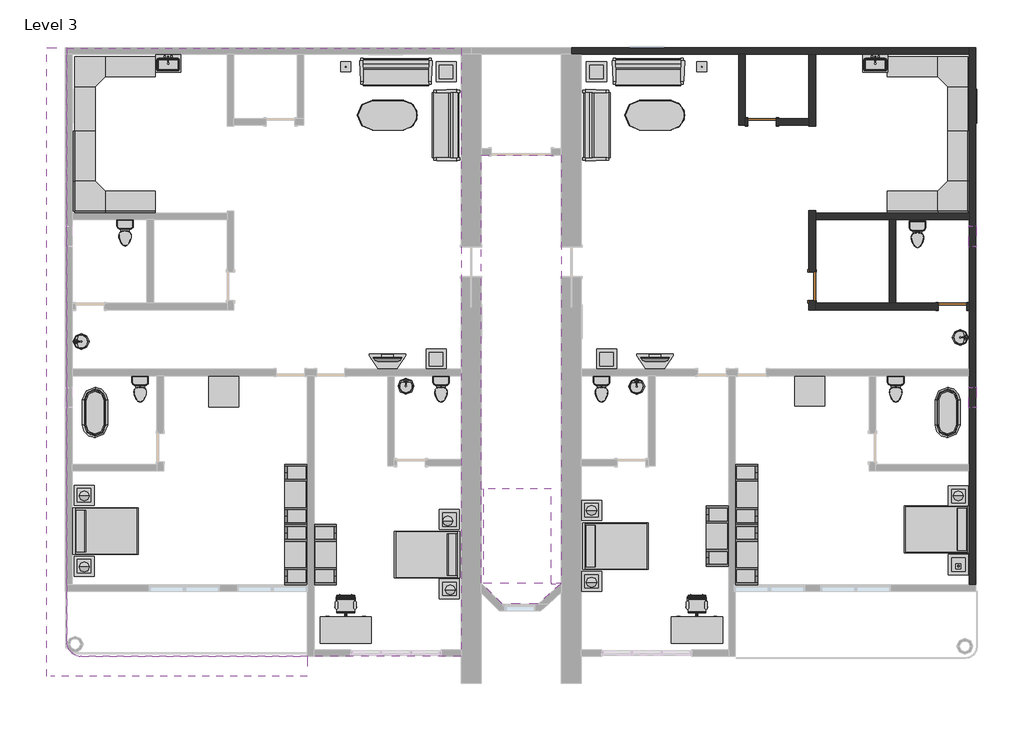
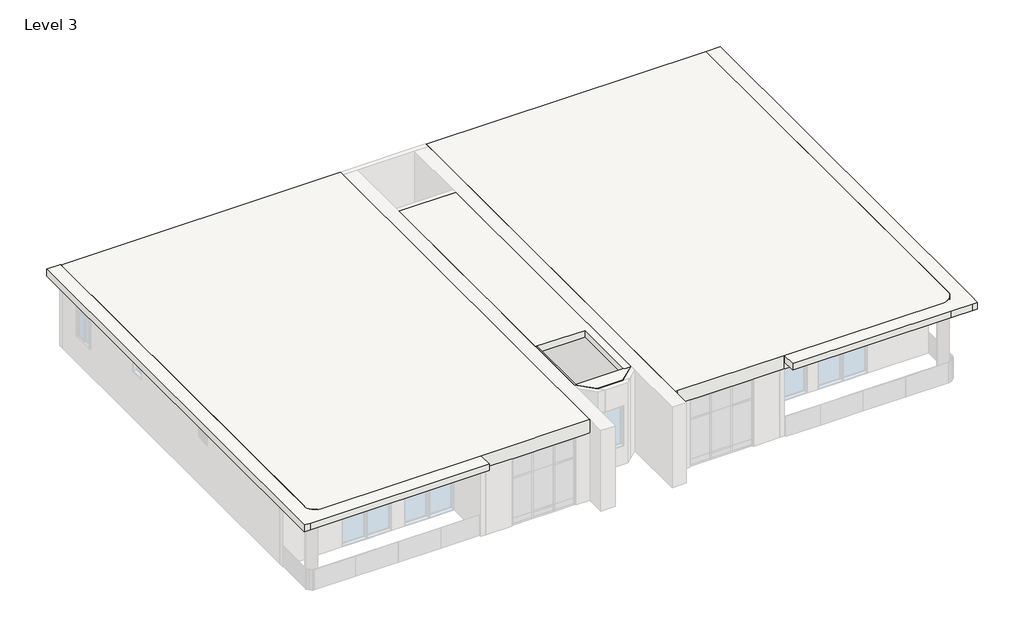
# One storey, part 3 of 3: 42 furniture elements, 14 flow terminals, 10 light fixtures, 9 walls, 4 slabs, 3 doors, 3 windows.
"""IFC4 building model written with IfcOpenShell, lengths in millimetres."""

from ifc_helpers import new_model, si_unit, point, frame, frame_2d, origin, place, context, project, spatial, polyline, circle_curve, trimmed, segment, composite_curve, outline, extrude, faceted_brep, transform, mapped, element, save
from components import door_2703ae13, door_10fd3a06, flow_terminal_38af2918, flow_terminal_d49f872f, toilet_domestic_3d_toilet_domestic_3d_f7549cf7, toilet_domestic_3d_toilet_domestic_3d_183bbd19, flow_terminal_b374fae2, furniture_07436f11, furniture_096e7f55, chair_task_arms_chair_task_arms_fa5a08ef, furniture_072f6425, furniture_cf0b6580, furniture_aff9b2fb, furniture_56245f3a, tv_stand_tv_stand_6ce107e5, furniture_b5c51a22, furniture_2c34a4f9, furniture_4d44e21c, furniture_45e3acac, light_fixture_100w_120v_8564026f, table_lamp_hemispheric_60w_120v_02721d88, window_0038ecf3, window_54100e87

model = new_model("IFC4")

# Units and contexts
model_context = context("Model", 3, world=origin())
ifc_project = project(units=[si_unit("LENGTHUNIT", "METRE", prefix="MILLI")], contexts=[model_context])

# Site, building, storey
site = spatial("IfcSite", under=ifc_project)
building = spatial("IfcBuilding", under=site)
storey = spatial("IfcBuildingStorey", under=building, Name="Level 3", Elevation=7315.2)

# Doors
placement = place(None, origin())
door_shape = door_2703ae13(model_context)
element("IfcDoor", 1, ObjectType="Door-Single-Panel.0001 : 34\" x 80\"", at=placement, inside=storey, context=model_context, shape_type="MappedRepresentation", body=[
    mapped(door_shape, transform((2528.3512296, 9464.0758558, 7315.2), x_axis=(-1.0, 0.0, 0.0), y_axis=(0.0, -1.0, 0.0), z_axis=(0.0, 0.0, 1.0))),
])
door_2_shape = door_10fd3a06(model_context)
element("IfcDoor", 2, ObjectType="Door-Single-Panel.0001 : 34\" x 80\"", at=placement, inside=storey, context=model_context, shape_type="MappedRepresentation", body=[
    mapped(door_2_shape, transform((8319.5512296, 3850.6758558, 7315.2), x_axis=(1.0, 0.0, 0.0), y_axis=(0.0, 1.0, 0.0), z_axis=(0.0, 0.0, 1.0))),
])
element("IfcDoor", 3, ObjectType="Door-Single-Panel.0001 : 34\" x 80\"", at=placement, inside=storey, context=model_context, shape_type="MappedRepresentation", body=[
    mapped(door_2_shape, transform((4052.3512296, 4460.2758558, 7315.2), x_axis=(0.0, -1.0, 0.0), y_axis=(1.0, 0.0, 0.0), z_axis=(0.0, 0.0, 1.0))),
])

# Flow terminals
flow_terminal_shape = flow_terminal_38af2918(model_context)
element("IfcFlowTerminal", 4, ObjectType="Sink Kitchen-Single : 30\" x 21\"", at=placement, inside=storey, context=model_context, shape_type="MappedRepresentation", body=[
    mapped(flow_terminal_shape, transform((-15534.038011, 11239.7304546, 7315.2), x_axis=(1.0, 0.0, 0.0), y_axis=(0.0, 1.0, 0.0), z_axis=(0.0, 0.0, 1.0))),
])
element("IfcFlowTerminal", 5, ObjectType="Sink Kitchen-Single : 30\" x 21\"", at=placement, inside=storey, context=model_context, shape_type="MappedRepresentation", body=[
    mapped(flow_terminal_shape, transform((5954.361989, 11239.7304546, 7315.2), x_axis=(1.0, 0.0, 0.0), y_axis=(0.0, 1.0, 0.0), z_axis=(0.0, 0.0, 1.0))),
])
flow_terminal_2_shape = flow_terminal_d49f872f(model_context)
element("IfcFlowTerminal", 6, ObjectType="Sink Vanity-Round : 19\" x 19\"", at=placement, inside=storey, context=model_context, shape_type="MappedRepresentation", body=[
    mapped(flow_terminal_2_shape, transform((-18078.2570794, 2687.2241152, 7315.2), x_axis=(0.0, 1.0, 0.0), y_axis=(-1.0, 0.0, 0.0), z_axis=(0.0, 0.0, 1.0))),
])
element("IfcFlowTerminal", 7, ObjectType="Sink Vanity-Round : 19\" x 19\"", at=placement, inside=storey, context=model_context, shape_type="MappedRepresentation", body=[
    mapped(flow_terminal_2_shape, transform((8468.5749463, 3007.5275963, 7315.2), x_axis=(0.0, -1.0, 0.0), y_axis=(1.0, 0.0, 0.0), z_axis=(0.0, 0.0, 1.0))),
])
element("IfcFlowTerminal", 8, ObjectType="Sink Vanity-Round : 19\" x 19\"", at=placement, inside=storey, context=model_context, shape_type="MappedRepresentation", body=[
    mapped(flow_terminal_2_shape, transform((-8388.700511, 1341.8921141, 7315.2), x_axis=(1.0, 0.0, 0.0), y_axis=(0.0, 1.0, 0.0), z_axis=(0.0, 0.0, 1.0))),
])
element("IfcFlowTerminal", 9, ObjectType="Sink Vanity-Round : 19\" x 19\"", at=placement, inside=storey, context=model_context, shape_type="MappedRepresentation", body=[
    mapped(flow_terminal_2_shape, transform((-1378.300511, 1331.0855344, 7315.2), x_axis=(1.0, 0.0, 0.0), y_axis=(0.0, 1.0, 0.0), z_axis=(0.0, 0.0, 1.0))),
])
toilet_domestic_3d_toilet_domestic_3d_shape = toilet_domestic_3d_toilet_domestic_3d_f7549cf7(model_context)
toilet_domestic_3d_toilet_domestic_3d_2_shape = toilet_domestic_3d_toilet_domestic_3d_183bbd19(model_context)
element("IfcFlowTerminal", 10, ObjectType="Toilet-Domestic-3D : Toilet-Domestic-3D", at=placement, inside=storey, context=model_context, shape_type="MappedRepresentation", body=[
    mapped(toilet_domestic_3d_toilet_domestic_3d_shape, transform((6592.3512296, 1247.7798284, 7315.2), x_axis=(1.0, 0.0, 0.0), y_axis=(0.0, 1.0, 0.0), z_axis=(0.0, 0.0, 1.0))),
    mapped(toilet_domestic_3d_toilet_domestic_3d_2_shape, transform((6592.3512296, 1247.7798284, 7315.2), x_axis=(1.0, 0.0, 0.0), y_axis=(0.0, 1.0, 0.0), z_axis=(0.0, 0.0, 1.0))),
])
element("IfcFlowTerminal", 11, ObjectType="Toilet-Domestic-3D : Toilet-Domestic-3D", at=placement, inside=storey, context=model_context, shape_type="MappedRepresentation", body=[
    mapped(toilet_domestic_3d_toilet_domestic_3d_shape, transform((-2348.4487704, 1247.7798284, 7315.2), x_axis=(1.0, 0.0, 0.0), y_axis=(0.0, 1.0, 0.0), z_axis=(0.0, 0.0, 1.0))),
    mapped(toilet_domestic_3d_toilet_domestic_3d_2_shape, transform((-2348.4487704, 1247.7798284, 7315.2), x_axis=(1.0, 0.0, 0.0), y_axis=(0.0, 1.0, 0.0), z_axis=(0.0, 0.0, 1.0))),
])
element("IfcFlowTerminal", 12, ObjectType="Toilet-Domestic-3D : Toilet-Domestic-3D", at=placement, inside=storey, context=model_context, shape_type="MappedRepresentation", body=[
    mapped(toilet_domestic_3d_toilet_domestic_3d_shape, transform((-16369.2487704, 1247.7798284, 7315.2), x_axis=(1.0, 0.0, 0.0), y_axis=(0.0, 1.0, 0.0), z_axis=(0.0, 0.0, 1.0))),
    mapped(toilet_domestic_3d_toilet_domestic_3d_2_shape, transform((-16369.2487704, 1247.7798284, 7315.2), x_axis=(1.0, 0.0, 0.0), y_axis=(0.0, 1.0, 0.0), z_axis=(0.0, 0.0, 1.0))),
])
element("IfcFlowTerminal", 13, ObjectType="Toilet-Domestic-3D : Toilet-Domestic-3D", at=placement, inside=storey, context=model_context, shape_type="MappedRepresentation", body=[
    mapped(toilet_domestic_3d_toilet_domestic_3d_shape, transform((-16826.4487704, 5997.5798284, 7315.2), x_axis=(1.0, 0.0, 0.0), y_axis=(0.0, 1.0, 0.0), z_axis=(0.0, 0.0, 1.0))),
    mapped(toilet_domestic_3d_toilet_domestic_3d_2_shape, transform((-16826.4487704, 5997.5798284, 7315.2), x_axis=(1.0, 0.0, 0.0), y_axis=(0.0, 1.0, 0.0), z_axis=(0.0, 0.0, 1.0))),
])
element("IfcFlowTerminal", 14, ObjectType="Toilet-Domestic-3D : Toilet-Domestic-3D", at=placement, inside=storey, context=model_context, shape_type="MappedRepresentation", body=[
    mapped(toilet_domestic_3d_toilet_domestic_3d_shape, transform((7252.7512296, 5946.7798284, 7315.2), x_axis=(1.0, 0.0, 0.0), y_axis=(0.0, 1.0, 0.0), z_axis=(0.0, 0.0, 1.0))),
    mapped(toilet_domestic_3d_toilet_domestic_3d_2_shape, transform((7252.7512296, 5946.7798284, 7315.2), x_axis=(1.0, 0.0, 0.0), y_axis=(0.0, 1.0, 0.0), z_axis=(0.0, 0.0, 1.0))),
])
element("IfcFlowTerminal", 15, ObjectType="Toilet-Domestic-3D : Toilet-Domestic-3D", at=placement, inside=storey, context=model_context, shape_type="MappedRepresentation", body=[
    mapped(toilet_domestic_3d_toilet_domestic_3d_shape, transform((-7225.2487704, 1247.7798284, 7315.2), x_axis=(1.0, 0.0, 0.0), y_axis=(0.0, 1.0, 0.0), z_axis=(0.0, 0.0, 1.0))),
    mapped(toilet_domestic_3d_toilet_domestic_3d_2_shape, transform((-7225.2487704, 1247.7798284, 7315.2), x_axis=(1.0, 0.0, 0.0), y_axis=(0.0, 1.0, 0.0), z_axis=(0.0, 0.0, 1.0))),
])
flow_terminal_3_shape = flow_terminal_b374fae2(model_context)
element("IfcFlowTerminal", 16, ObjectType="Tub-Free Standing-3D : 30\" x 60\"", at=placement, inside=storey, context=model_context, shape_type="MappedRepresentation", body=[
    mapped(flow_terminal_3_shape, transform((-17740.8487704, 624.8758558, 7315.2), x_axis=(1.0, 0.0, 0.0), y_axis=(0.0, 1.0, 0.0), z_axis=(0.0, 0.0, 1.0))),
])
element("IfcFlowTerminal", 17, ObjectType="Tub-Free Standing-3D : 30\" x 60\"", at=placement, inside=storey, context=model_context, shape_type="MappedRepresentation", body=[
    mapped(flow_terminal_3_shape, transform((8167.1512296, 624.8758558, 7315.2), x_axis=(1.0, 0.0, 0.0), y_axis=(0.0, 1.0, 0.0), z_axis=(0.0, 0.0, 1.0))),
])

# Furniture
furniture_shape = furniture_07436f11(model_context)
element("IfcFurniture", 18, ObjectType="96\" x 96\"", at=placement, inside=storey, context=model_context, shape_type="MappedRepresentation", body=[
    mapped(furniture_shape, transform((-18269.5170182, 11991.0988634, 7315.2), x_axis=(1.0, 0.0, 0.0), y_axis=(0.0, 1.0, 0.0), z_axis=(0.0, 0.0, 1.0))),
])
element("IfcFurniture", 19, ObjectType="96\" x 96\"", at=placement, inside=storey, context=model_context, shape_type="MappedRepresentation", body=[
    mapped(furniture_shape, transform((9322.5742372, 11364.3441035, 7315.2), x_axis=(0.0, -1.0, 0.0), y_axis=(1.0, 0.0, 0.0), z_axis=(0.0, 0.0, 1.0))),
])
furniture_2_shape = furniture_096e7f55(model_context)
element("IfcFurniture", 20, ObjectType="Bed-Shaker : Double 56\" x 78\"", at=placement, inside=storey, context=model_context, shape_type="MappedRepresentation", body=[
    mapped(furniture_2_shape, transform((-18401.2487704, -2962.8741442, 7315.2), x_axis=(0.0, 1.0, 0.0), y_axis=(-1.0, 0.0, 0.0), z_axis=(0.0, 0.0, 1.0))),
])
element("IfcFurniture", 21, ObjectType="Bed-Shaker : Double 56\" x 78\"", at=placement, inside=storey, context=model_context, shape_type="MappedRepresentation", body=[
    mapped(furniture_2_shape, transform((-6666.4487704, -3712.1741442, 7315.2), x_axis=(0.0, -1.0, 0.0), y_axis=(1.0, 0.0, 0.0), z_axis=(0.0, 0.0, 1.0))),
])
element("IfcFurniture", 22, ObjectType="Bed-Shaker : Double 56\" x 78\"", at=placement, inside=storey, context=model_context, shape_type="MappedRepresentation", body=[
    mapped(furniture_2_shape, transform((-2907.2487704, -3420.0741442, 7315.2), x_axis=(0.0, 1.0, 0.0), y_axis=(-1.0, 0.0, 0.0), z_axis=(0.0, 0.0, 1.0))),
])
element("IfcFurniture", 23, ObjectType="Bed-Shaker : Double 56\" x 78\"", at=placement, inside=storey, context=model_context, shape_type="MappedRepresentation", body=[
    mapped(furniture_2_shape, transform((8827.5512296, -2950.1741442, 7315.2), x_axis=(0.0, -1.0, 0.0), y_axis=(1.0, 0.0, 0.0), z_axis=(0.0, 0.0, 1.0))),
])
chair_task_arms_chair_task_arms_shape = chair_task_arms_chair_task_arms_fa5a08ef(model_context)
element("IfcFurniture", 24, ObjectType="Chair-Task Arms : Chair-Task Arms", at=placement, inside=storey, context=model_context, shape_type="MappedRepresentation", body=[
    mapped(chair_task_arms_chair_task_arms_shape, transform((688.1420493, -5184.3566833, 7315.2), x_axis=(-1.0, 0.0, 0.0), y_axis=(0.0, -1.0, 0.0), z_axis=(0.0, 0.0, 1.0))),
])
element("IfcFurniture", 25, ObjectType="Chair-Task Arms : Chair-Task Arms", at=placement, inside=storey, context=model_context, shape_type="MappedRepresentation", body=[
    mapped(chair_task_arms_chair_task_arms_shape, transform((-9979.8579507, -5184.3566833, 7315.2), x_axis=(-1.0, 0.0, 0.0), y_axis=(0.0, -1.0, 0.0), z_axis=(0.0, 0.0, 1.0))),
])
furniture_3_shape = furniture_072f6425(model_context)
element("IfcFurniture", 26, ObjectType="Desk : 60\" x 30\"", at=placement, inside=storey, context=model_context, shape_type="MappedRepresentation", body=[
    mapped(furniture_3_shape, transform((-10882.8487704, -6371.702585, 7315.2), x_axis=(1.0, 0.0, 0.0), y_axis=(0.0, 1.0, 0.0), z_axis=(0.0, 0.0, 1.0))),
])
element("IfcFurniture", 27, ObjectType="Desk : 60\" x 30\"", at=placement, inside=storey, context=model_context, shape_type="MappedRepresentation", body=[
    mapped(furniture_3_shape, transform((-214.8487704, -6371.702585, 7315.2), x_axis=(1.0, 0.0, 0.0), y_axis=(0.0, 1.0, 0.0), z_axis=(0.0, 0.0, 1.0))),
])
furniture_4_shape = furniture_cf0b6580(model_context)
element("IfcFurniture", 28, ObjectType="Entertainment Center : 72\" x 72\" x 24\"", at=placement, inside=storey, context=model_context, shape_type="MappedRepresentation", body=[
    mapped(furniture_4_shape, transform((1613.9512296, -3134.3241442, 7315.2), x_axis=(0.0, -1.0, 0.0), y_axis=(1.0, 0.0, 0.0), z_axis=(0.0, 0.0, 1.0))),
])
element("IfcFurniture", 29, ObjectType="Entertainment Center : 72\" x 72\" x 24\"", at=placement, inside=storey, context=model_context, shape_type="MappedRepresentation", body=[
    mapped(furniture_4_shape, transform((1613.9512296, -3693.1241442, 7315.2), x_axis=(0.0, 1.0, 0.0), y_axis=(-1.0, 0.0, 0.0), z_axis=(0.0, 0.0, 1.0))),
])
element("IfcFurniture", 30, ObjectType="Entertainment Center : 72\" x 72\" x 24\"", at=placement, inside=storey, context=model_context, shape_type="MappedRepresentation", body=[
    mapped(furniture_4_shape, transform((1613.9512296, -1864.3241442, 7315.2), x_axis=(0.0, 1.0, 0.0), y_axis=(-1.0, 0.0, 0.0), z_axis=(0.0, 0.0, 1.0))),
])
element("IfcFurniture", 31, ObjectType="Entertainment Center : 72\" x 72\" x 24\"", at=placement, inside=storey, context=model_context, shape_type="MappedRepresentation", body=[
    mapped(furniture_4_shape, transform((-11187.6487704, -3693.1241442, 7315.2), x_axis=(0.0, -1.0, 0.0), y_axis=(1.0, 0.0, 0.0), z_axis=(0.0, 0.0, 1.0))),
])
element("IfcFurniture", 32, ObjectType="Entertainment Center : 72\" x 72\" x 24\"", at=placement, inside=storey, context=model_context, shape_type="MappedRepresentation", body=[
    mapped(furniture_4_shape, transform((-11187.6487704, -1864.3241442, 7315.2), x_axis=(0.0, -1.0, 0.0), y_axis=(1.0, 0.0, 0.0), z_axis=(0.0, 0.0, 1.0))),
])
element("IfcFurniture", 33, ObjectType="Entertainment Center : 72\" x 72\" x 24\"", at=placement, inside=storey, context=model_context, shape_type="MappedRepresentation", body=[
    mapped(furniture_4_shape, transform((-11187.6487704, -3693.1241442, 7315.2), x_axis=(0.0, 1.0, 0.0), y_axis=(-1.0, 0.0, 0.0), z_axis=(0.0, 0.0, 1.0))),
])
furniture_5_shape = furniture_aff9b2fb(model_context)
element("IfcFurniture", 34, ObjectType="Sofa-Pensi : 84\"", at=placement, inside=storey, context=model_context, shape_type="MappedRepresentation", body=[
    mapped(furniture_5_shape, transform((-8875.4550204, 10710.9660197, 7315.2), x_axis=(1.0, 0.0, 0.0), y_axis=(0.0, 1.0, 0.0), z_axis=(0.0, 0.0, 1.0))),
])
element("IfcFurniture", 35, ObjectType="Sofa-Pensi : 84\"", at=placement, inside=storey, context=model_context, shape_type="MappedRepresentation", body=[
    mapped(furniture_5_shape, transform((-7349.9586065, 9641.0821058, 7315.2), x_axis=(0.0, -1.0, 0.0), y_axis=(1.0, 0.0, 0.0), z_axis=(0.0, 0.0, 1.0))),
])
element("IfcFurniture", 36, ObjectType="Sofa-Pensi : 84\"", at=placement, inside=storey, context=model_context, shape_type="MappedRepresentation", body=[
    mapped(furniture_5_shape, transform((-2223.7389343, 9083.8696058, 7315.2), x_axis=(0.0, 1.0, 0.0), y_axis=(-1.0, 0.0, 0.0), z_axis=(0.0, 0.0, 1.0))),
])
element("IfcFurniture", 37, ObjectType="Sofa-Pensi : 84\"", at=placement, inside=storey, context=model_context, shape_type="MappedRepresentation", body=[
    mapped(furniture_5_shape, transform((-1204.6550204, 10710.9660197, 7315.2), x_axis=(1.0, 0.0, 0.0), y_axis=(0.0, 1.0, 0.0), z_axis=(0.0, 0.0, 1.0))),
])
furniture_6_shape = furniture_56245f3a(model_context)
element("IfcFurniture", 38, ObjectType="TV - Flat Screen : 32\"", at=placement, inside=storey, context=model_context, shape_type="MappedRepresentation", body=[
    mapped(furniture_6_shape, transform((-8854.7932846, 2232.8144794, 8229.6), x_axis=(-1.0, 0.0, 0.0), y_axis=(0.0, -1.0, 0.0), z_axis=(0.0, 0.0, 1.0))),
])
element("IfcFurniture", 39, ObjectType="TV - Flat Screen : 32\"", at=placement, inside=storey, context=model_context, shape_type="MappedRepresentation", body=[
    mapped(furniture_6_shape, transform((-726.7932846, 2232.8144794, 8229.6), x_axis=(-1.0, 0.0, 0.0), y_axis=(0.0, -1.0, 0.0), z_axis=(0.0, 0.0, 1.0))),
])
tv_stand_tv_stand_shape = tv_stand_tv_stand_6ce107e5(model_context)
element("IfcFurniture", 40, ObjectType="TV Stand : TV Stand", at=placement, inside=storey, context=model_context, shape_type="MappedRepresentation", body=[
    mapped(tv_stand_tv_stand_shape, transform((-8725.6607683, 1945.6758558, 7315.2), x_axis=(-1.0, 0.0, 0.0), y_axis=(0.0, -1.0, 0.0), z_axis=(0.0, 0.0, 1.0))),
])
element("IfcFurniture", 41, ObjectType="TV Stand : TV Stand", at=placement, inside=storey, context=model_context, shape_type="MappedRepresentation", body=[
    mapped(tv_stand_tv_stand_shape, transform((-597.6607683, 1945.6758558, 7315.2), x_axis=(-1.0, 0.0, 0.0), y_axis=(0.0, -1.0, 0.0), z_axis=(0.0, 0.0, 1.0))),
])
furniture_7_shape = furniture_b5c51a22(model_context)
element("IfcFurniture", 42, ObjectType="Table-Coffee : 24\" x 24\" x 24\"", at=placement, inside=storey, context=model_context, shape_type="MappedRepresentation", body=[
    mapped(furniture_7_shape, transform((-7091.1145371, 10892.864778, 7315.2), x_axis=(1.0, 0.0, 0.0), y_axis=(0.0, 1.0, 0.0), z_axis=(0.0, 0.0, 1.0))),
])
element("IfcFurniture", 43, ObjectType="Table-Coffee : 24\" x 24\" x 24\"", at=placement, inside=storey, context=model_context, shape_type="MappedRepresentation", body=[
    mapped(furniture_7_shape, transform((-2519.1145371, 10892.864778, 7315.2), x_axis=(1.0, 0.0, 0.0), y_axis=(0.0, 1.0, 0.0), z_axis=(0.0, 0.0, 1.0))),
])
element("IfcFurniture", 44, ObjectType="Table-Coffee : 24\" x 24\" x 24\"", at=placement, inside=storey, context=model_context, shape_type="MappedRepresentation", body=[
    mapped(furniture_7_shape, transform((-7395.9145371, 2155.264778, 7315.2), x_axis=(1.0, 0.0, 0.0), y_axis=(0.0, 1.0, 0.0), z_axis=(0.0, 0.0, 1.0))),
])
element("IfcFurniture", 45, ObjectType="Table-Coffee : 24\" x 24\" x 24\"", at=placement, inside=storey, context=model_context, shape_type="MappedRepresentation", body=[
    mapped(furniture_7_shape, transform((-2214.3145371, 2155.264778, 7315.2), x_axis=(1.0, 0.0, 0.0), y_axis=(0.0, 1.0, 0.0), z_axis=(0.0, 0.0, 1.0))),
])
element("IfcFurniture", 46, ObjectType="Table-Coffee : 24\" x 24\" x 24\"", at=placement, inside=storey, context=model_context, shape_type="MappedRepresentation", body=[
    mapped(furniture_7_shape, transform((-2671.5145371, -4601.135222, 7315.2), x_axis=(1.0, 0.0, 0.0), y_axis=(0.0, 1.0, 0.0), z_axis=(0.0, 0.0, 1.0))),
])
element("IfcFurniture", 47, ObjectType="Table-Coffee : 24\" x 24\" x 24\"", at=placement, inside=storey, context=model_context, shape_type="MappedRepresentation", body=[
    mapped(furniture_7_shape, transform((-18089.3145371, -4143.935222, 7315.2), x_axis=(1.0, 0.0, 0.0), y_axis=(0.0, 1.0, 0.0), z_axis=(0.0, 0.0, 1.0))),
])
element("IfcFurniture", 48, ObjectType="Table-Coffee : 24\" x 24\" x 24\"", at=placement, inside=storey, context=model_context, shape_type="MappedRepresentation", body=[
    mapped(furniture_7_shape, transform((-18089.3145371, -1984.935222, 7315.2), x_axis=(1.0, 0.0, 0.0), y_axis=(0.0, 1.0, 0.0), z_axis=(0.0, 0.0, 1.0))),
])
element("IfcFurniture", 49, ObjectType="Table-Coffee : 24\" x 24\" x 24\"", at=placement, inside=storey, context=model_context, shape_type="MappedRepresentation", body=[
    mapped(furniture_7_shape, transform((-2671.5145371, -2442.135222, 7315.2), x_axis=(1.0, 0.0, 0.0), y_axis=(0.0, 1.0, 0.0), z_axis=(0.0, 0.0, 1.0))),
])
element("IfcFurniture", 50, ObjectType="Table-Coffee : 24\" x 24\" x 24\"", at=placement, inside=storey, context=model_context, shape_type="MappedRepresentation", body=[
    mapped(furniture_7_shape, transform((8479.0854629, -4093.135222, 7315.2), x_axis=(1.0, 0.0, 0.0), y_axis=(0.0, 1.0, 0.0), z_axis=(0.0, 0.0, 1.0))),
])
element("IfcFurniture", 51, ObjectType="Table-Coffee : 24\" x 24\" x 24\"", at=placement, inside=storey, context=model_context, shape_type="MappedRepresentation", body=[
    mapped(furniture_7_shape, transform((8479.0854629, -2010.335222, 7315.2), x_axis=(1.0, 0.0, 0.0), y_axis=(0.0, 1.0, 0.0), z_axis=(0.0, 0.0, 1.0))),
])
element("IfcFurniture", 52, ObjectType="Table-Coffee : 24\" x 24\" x 24\"", at=placement, inside=storey, context=model_context, shape_type="MappedRepresentation", body=[
    mapped(furniture_7_shape, transform((-6989.5145371, -4832.0414601, 7315.2), x_axis=(1.0, 0.0, 0.0), y_axis=(0.0, 1.0, 0.0), z_axis=(0.0, 0.0, 1.0))),
])
element("IfcFurniture", 53, ObjectType="Table-Coffee : 24\" x 24\" x 24\"", at=placement, inside=storey, context=model_context, shape_type="MappedRepresentation", body=[
    mapped(furniture_7_shape, transform((-6989.5145371, -2723.8414601, 7315.2), x_axis=(1.0, 0.0, 0.0), y_axis=(0.0, 1.0, 0.0), z_axis=(0.0, 0.0, 1.0))),
])
furniture_8_shape = furniture_2c34a4f9(model_context)
element("IfcFurniture", 54, ObjectType="Table-Dining Oval : 36\" x 72\"", at=placement, inside=storey, context=model_context, shape_type="MappedRepresentation", body=[
    mapped(furniture_8_shape, transform((-8449.0290983, 10025.3742164, 7315.2), x_axis=(1.0, 0.0, 0.0), y_axis=(0.0, 1.0, 0.0), z_axis=(0.0, 0.0, 1.0))),
])
element("IfcFurniture", 55, ObjectType="Table-Dining Oval : 36\" x 72\"", at=placement, inside=storey, context=model_context, shape_type="MappedRepresentation", body=[
    mapped(furniture_8_shape, transform((-321.0290983, 10025.3742164, 7315.2), x_axis=(1.0, 0.0, 0.0), y_axis=(0.0, 1.0, 0.0), z_axis=(0.0, 0.0, 1.0))),
])
furniture_9_shape = furniture_4d44e21c(model_context)
element("IfcFurniture", 56, ObjectType="Table-Rectangular : 36\" x 36\"", at=placement, inside=storey, context=model_context, shape_type="MappedRepresentation", body=[
    mapped(furniture_9_shape, transform((-13829.2487704, 1259.8758558, 7315.2), x_axis=(1.0, 0.0, 0.0), y_axis=(0.0, 1.0, 0.0), z_axis=(0.0, 0.0, 1.0))),
])
element("IfcFurniture", 57, ObjectType="Table-Rectangular : 36\" x 36\"", at=placement, inside=storey, context=model_context, shape_type="MappedRepresentation", body=[
    mapped(furniture_9_shape, transform((3976.1512296, 1285.2758558, 7315.2), x_axis=(1.0, 0.0, 0.0), y_axis=(0.0, 1.0, 0.0), z_axis=(0.0, 0.0, 1.0))),
])
furniture_10_shape = furniture_45e3acac(model_context)
element("IfcFurniture", 58, ObjectType="Work Station Cubicle : 96\" x 96\"", at=placement, inside=storey, context=model_context, shape_type="MappedRepresentation", body=[
    mapped(furniture_10_shape, transform((-18896.271778, 6827.207608, 7315.2), x_axis=(0.0, 1.0, 0.0), y_axis=(-1.0, 0.0, 0.0), z_axis=(0.0, 0.0, 1.0))),
])
element("IfcFurniture", 59, ObjectType="Work Station Cubicle : 96\" x 96\"", at=placement, inside=storey, context=model_context, shape_type="MappedRepresentation", body=[
    mapped(furniture_10_shape, transform((8695.8194774, 6200.4528481, 7315.2), x_axis=(-1.0, 0.0, 0.0), y_axis=(0.0, -1.0, 0.0), z_axis=(0.0, 0.0, 1.0))),
])

# Light fixtures
light_fixture_100w_120v_shape = light_fixture_100w_120v_8564026f(model_context)
element("IfcLightFixture", 60, ObjectType="100W - 120V", at=placement, inside=storey, context=model_context, shape_type="MappedRepresentation", body=[
    mapped(light_fixture_100w_120v_shape, transform((-10120.8487704, 11140.4758558, 7315.2), x_axis=(1.0, 0.0, 0.0), y_axis=(0.0, 1.0, 0.0), z_axis=(0.0, 0.0, 1.0))),
])
element("IfcLightFixture", 61, ObjectType="100W - 120V", at=placement, inside=storey, context=model_context, shape_type="MappedRepresentation", body=[
    mapped(light_fixture_100w_120v_shape, transform((699.5512296, 11140.4758558, 7315.2), x_axis=(1.0, 0.0, 0.0), y_axis=(0.0, 1.0, 0.0), z_axis=(0.0, 0.0, 1.0))),
])
table_lamp_hemispheric_60w_120v_shape = table_lamp_hemispheric_60w_120v_02721d88(model_context)
element("IfcLightFixture", 62, ObjectType="Table Lamp - Hemispheric : 60W - 120V", at=placement, inside=storey, context=model_context, shape_type="MappedRepresentation", body=[
    mapped(table_lamp_hemispheric_60w_120v_shape, transform((-18071.0487704, -1915.1241442, 7924.8), x_axis=(1.0, 0.0, 0.0), y_axis=(0.0, 1.0, 0.0), z_axis=(0.0, 0.0, 1.0))),
])
element("IfcLightFixture", 63, ObjectType="Table Lamp - Hemispheric : 60W - 120V", at=placement, inside=storey, context=model_context, shape_type="MappedRepresentation", body=[
    mapped(table_lamp_hemispheric_60w_120v_shape, transform((-7022.0487704, -2666.7303823, 7924.8), x_axis=(1.0, 0.0, 0.0), y_axis=(0.0, 1.0, 0.0), z_axis=(0.0, 0.0, 1.0))),
])
element("IfcLightFixture", 64, ObjectType="Table Lamp - Hemispheric : 60W - 120V", at=placement, inside=storey, context=model_context, shape_type="MappedRepresentation", body=[
    mapped(table_lamp_hemispheric_60w_120v_shape, transform((-2653.2487704, -2346.9241442, 7924.8), x_axis=(1.0, 0.0, 0.0), y_axis=(0.0, 1.0, 0.0), z_axis=(0.0, 0.0, 1.0))),
])
element("IfcLightFixture", 65, ObjectType="Table Lamp - Hemispheric : 60W - 120V", at=placement, inside=storey, context=model_context, shape_type="MappedRepresentation", body=[
    mapped(table_lamp_hemispheric_60w_120v_shape, transform((8497.3512296, -4048.7241442, 8229.6), x_axis=(1.0, 0.0, 0.0), y_axis=(0.0, 1.0, 0.0), z_axis=(0.0, 0.0, 1.0))),
])
element("IfcLightFixture", 66, ObjectType="Table Lamp - Hemispheric : 60W - 120V", at=placement, inside=storey, context=model_context, shape_type="MappedRepresentation", body=[
    mapped(table_lamp_hemispheric_60w_120v_shape, transform((8497.3512296, -1915.1241442, 7924.8), x_axis=(1.0, 0.0, 0.0), y_axis=(0.0, 1.0, 0.0), z_axis=(0.0, 0.0, 1.0))),
])
element("IfcLightFixture", 67, ObjectType="Table Lamp - Hemispheric : 60W - 120V", at=placement, inside=storey, context=model_context, shape_type="MappedRepresentation", body=[
    mapped(table_lamp_hemispheric_60w_120v_shape, transform((-2653.2487704, -4531.3241442, 7924.8), x_axis=(1.0, 0.0, 0.0), y_axis=(0.0, 1.0, 0.0), z_axis=(0.0, 0.0, 1.0))),
])
element("IfcLightFixture", 68, ObjectType="Table Lamp - Hemispheric : 60W - 120V", at=placement, inside=storey, context=model_context, shape_type="MappedRepresentation", body=[
    mapped(table_lamp_hemispheric_60w_120v_shape, transform((-6945.8487704, -4762.2303823, 7924.8), x_axis=(1.0, 0.0, 0.0), y_axis=(0.0, 1.0, 0.0), z_axis=(0.0, 0.0, 1.0))),
])
element("IfcLightFixture", 69, ObjectType="Table Lamp - Hemispheric : 60W - 120V", at=placement, inside=storey, context=model_context, shape_type="MappedRepresentation", body=[
    mapped(table_lamp_hemispheric_60w_120v_shape, transform((-18071.0487704, -4074.1241442, 7924.8), x_axis=(1.0, 0.0, 0.0), y_axis=(0.0, 1.0, 0.0), z_axis=(0.0, 0.0, 1.0))),
])

# Slabs
element("IfcSlab", 70, ObjectType="Generic - 12\" cream", at=placement, inside=storey, context=model_context, shape_type="SweptSolid", body=[
    extrude(outline(composite_curve([segment(polyline([(-6615.6487704, 11699.2758558), (-6615.6487704, -6791.9241442), (-11289.2487704, -6791.9241442), (-18147.2487704, -6791.9241442)]), True, "CONTINUOUS"), segment(trimmed(circle_curve(frame_2d((-18147.2487704, -6334.7241442)), 457.2), [point((-18147.2487704, -6791.9241442))], [point((-18604.4487704, -6334.7241442))], False, "CARTESIAN"), True, "CONTINUOUS"), segment(polyline([(-18604.4487704, -6334.7241442), (-18604.4487704, 11699.2758558), (-6615.6487704, 11699.2758558)]), True, "CONTINUOUS")], self_intersect=False)), frame((0.0, 0.0, 10363.2), z_axis=(0.0, 0.0, 1.0), x_axis=(1.0, 0.0, 0.0)), (0.0, 0.0, 1.0), 609.6),
    extrude(outline(composite_curve([segment(trimmed(circle_curve(frame_2d((8518.1543381, -6277.3874522)), 514.536692), [point((9030.7512296, -6322.0241442))], [point((8518.1543381, -6791.9241442))], False, "CARTESIAN"), True, "CONTINUOUS"), segment(polyline([(8518.1543381, -6791.9241442), (1715.5512296, -6791.9241442), (-2856.4487704, -6791.9241442), (-2958.0487704, -6791.9241442), (-2958.0487704, 11699.2758558), (9030.7512296, 11699.2758558), (9030.7512296, -6322.0241442)]), True, "CONTINUOUS")], self_intersect=False)), frame((0.0, 0.0, 10363.2), z_axis=(0.0, 0.0, 1.0), x_axis=(1.0, 0.0, 0.0)), (0.0, 0.0, 1.0), 609.6),
])
element("IfcSlab", 71, ObjectType="Generic - 12\" white", at=placement, inside=storey, context=model_context, shape_type="SweptSolid", body=[
    extrude(outline(composite_curve([segment(polyline([(9640.3512296, 11699.2758558), (9640.3512296, -6931.6241442), (9640.3512296, -7401.5241442), (9437.1512296, -7401.5241442), (8518.1543381, -7401.5241442), (1715.5512296, -7401.5241442), (1715.5512296, -6791.9241442), (8518.1543381, -6791.9241442)]), True, "CONTINUOUS"), segment(trimmed(circle_curve(frame_2d((8518.1543381, -6277.3874522)), 514.536692), [point((8518.1543381, -6791.9241442))], [point((9030.7512296, -6322.0241442))], True, "CARTESIAN"), True, "CONTINUOUS"), segment(polyline([(9030.7512296, -6322.0241442), (9030.7512296, 11699.2758558), (9640.3512296, 11699.2758558)]), True, "CONTINUOUS")], self_intersect=False)), frame((0.0, 0.0, 10668.0), z_axis=(0.0, 0.0, 1.0), x_axis=(1.0, 0.0, 0.0)), (0.0, 0.0, 1.0), 304.8),
    extrude(outline(composite_curve([segment(polyline([(-18604.4487704, 11724.6758558), (-18604.4487704, -6334.7241442)]), True, "CONTINUOUS"), segment(trimmed(circle_curve(frame_2d((-18147.2487704, -6334.7241442)), 457.2), [point((-18604.4487704, -6334.7241442))], [point((-18147.2487704, -6791.9241442))], True, "CARTESIAN"), True, "CONTINUOUS"), segment(polyline([(-18147.2487704, -6791.9241442), (-11289.2487704, -6791.9241442), (-11289.2487704, -7401.5241442), (-18960.0487704, -7401.5241442), (-19214.0487704, -7401.5241442), (-19214.0487704, 11724.6758558), (-18604.4487704, 11724.6758558)]), True, "CONTINUOUS")], self_intersect=False)), frame((0.0, 0.0, 10668.0), z_axis=(0.0, 0.0, 1.0), x_axis=(1.0, 0.0, 0.0)), (0.0, 0.0, 1.0), 304.8),
])
element("IfcSlab", 72, ObjectType="Generic - 12\" white", at=placement, inside=storey, context=model_context, shape_type="SweptSolid", body=[
    extrude(outline(polyline([(-3573.9987704, 8448.0758558), (-3573.9987704, -1691.5549149), (-3573.9987704, -4572.9908503), (-3878.7987704, -4572.9908503), (-3878.7987704, -1691.5549149), (-6006.0487704, -1691.5549149), (-6006.0487704, 8448.0758558), (-3573.9987704, 8448.0758558)])), frame((0.0, 0.0, 10668.0), z_axis=(0.0, 0.0, 1.0), x_axis=(1.0, 0.0, 0.0)), (0.0, 0.0, 1.0), 304.8),
])
element("IfcSlab", 73, ObjectType="Generic - 12\" white", at=placement, inside=storey, context=model_context, shape_type="SweptSolid", body=[
    extrude(outline(polyline([(-5940.8822214, -1691.5549149), (-5940.8822214, -4554.2130548), (-3874.1153195, -4554.2130548), (-3874.1153195, -4579.6130548), (-3594.7153195, -4579.6130548), (-4277.1570449, -5188.2185522), (-5369.3570449, -5188.2185522), (-5997.9749734, -4559.6006237), (-5997.9749734, -1691.5549149), (-5940.8822214, -1691.5549149)])), frame((0.0, 0.0, 10668.0), z_axis=(0.0, 0.0, 1.0), x_axis=(1.0, 0.0, 0.0)), (0.0, 0.0, 1.0), 304.8),
])

# Walls
element("IfcWall", 74, ObjectType="Generic - 8\" cream", at=placement, inside=storey, context=model_context, shape_type="Brep", body=[
    faceted_brep([(8827.5512296, 11724.6758558, 7315.2), (8827.5512296, 11521.4758558, 7315.2), (8827.5512296, 6695.4758558, 7315.2), (8827.5512296, 6492.2758558, 7315.2), (8827.5512296, 3952.2758558, 7315.2), (8827.5512296, 3749.0758558, 7315.2), (8827.5512296, 1945.6758558, 7315.2), (8827.5512296, 1742.4758558, 7315.2), (8827.5512296, -949.9241442, 7315.2), (8827.5512296, -1153.1241442, 7315.2), (8827.5512296, -4607.5241442, 7315.2), (8827.5512296, -4607.5241442, 10363.2), (8827.5512296, -1153.1241442, 10363.2), (8827.5512296, -949.9241442, 10363.2), (8827.5512296, 1742.4758558, 10363.2), (8827.5512296, 1945.6758558, 10363.2), (8827.5512296, 3749.0758558, 10363.2), (8827.5512296, 3952.2758558, 10363.2), (8827.5512296, 6492.2758558, 10363.2), (8827.5512296, 6695.4758558, 10363.2), (8827.5512296, 11521.4758558, 10363.2), (8827.5512296, 11724.6758558, 10363.2), (8827.5512296, 10403.8758558, 8534.4), (8827.5512296, 10403.8758558, 9753.6), (8827.5512296, 9489.4758558, 9753.6), (8827.5512296, 9489.4758558, 8534.4), (8827.5512296, 777.2758558, 10058.4), (8827.5512296, 777.2758558, 9448.8), (8827.5512296, 1386.8758558, 9448.8), (8827.5512296, 1386.8758558, 10058.4), (8827.5512296, 6289.0758558, 9448.8), (8827.5512296, 6289.0758558, 10058.4), (8827.5512296, 5679.4758558, 10058.4), (8827.5512296, 5679.4758558, 9448.8), (9030.7512296, -4607.5241442, 7315.2), (9030.7512296, 11724.6758558, 7315.2), (9030.7512296, 11724.6758558, 10363.2), (9030.7512296, -4607.5241442, 10363.2), (9030.7512296, 10403.8758558, 9753.6), (9030.7512296, 10403.8758558, 8534.4), (9030.7512296, 9489.4758558, 8534.4), (9030.7512296, 9489.4758558, 9753.6), (9030.7512296, 777.2758558, 9448.8), (9030.7512296, 777.2758558, 10058.4), (9030.7512296, 1386.8758558, 10058.4), (9030.7512296, 1386.8758558, 9448.8), (9030.7512296, 6289.0758558, 10058.4), (9030.7512296, 6289.0758558, 9448.8), (9030.7512296, 5679.4758558, 9448.8), (9030.7512296, 5679.4758558, 10058.4)], [[[0, 1, 2, 3, 4, 5, 6, 7, 8, 9, 10, 11, 12, 13, 14, 15, 16, 17, 18, 19, 20, 21], [22, 23, 24, 25], [26, 27, 28, 29], [30, 31, 32, 33]], [[34, 35, 36, 37], [38, 39, 40, 41], [42, 43, 44, 45], [46, 47, 48, 49]], [[10, 9, 8, 7, 6, 5, 4, 3, 2, 1, 0, 35, 34]], [[21, 20, 19, 18, 17, 16, 15, 14, 13, 12, 11, 37, 36]], [[0, 21, 36, 35]], [[11, 10, 34, 37]], [[39, 38, 23, 22]], [[40, 39, 22, 25]], [[41, 40, 25, 24]], [[38, 41, 24, 23]], [[26, 43, 42, 27]], [[27, 42, 45, 28]], [[28, 45, 44, 29]], [[43, 26, 29, 44]], [[46, 31, 30, 47]], [[47, 30, 33, 48]], [[48, 33, 32, 49]], [[31, 46, 49, 32]]]),
])
element("IfcWall", 75, ObjectType="Generic - 8\" cream", at=placement, inside=storey, context=model_context, shape_type="Brep", body=[
    faceted_brep([(3950.7512296, 11521.4758558, 7315.2), (3950.7512296, 9565.6758558, 7315.2), (3950.7512296, 9362.4758558, 7315.2), (3950.7512296, 9337.0758558, 7315.2), (3950.7512296, 9337.0758558, 10363.2), (3950.7512296, 9362.4758558, 10363.2), (3950.7512296, 9565.6758558, 10363.2), (3950.7512296, 11521.4758558, 10363.2), (4153.9512296, 11521.4758558, 7315.2), (4153.9512296, 11521.4758558, 10363.2), (4153.9512296, 9337.0758558, 10363.2), (4153.9512296, 9337.0758558, 7315.2)], [[[0, 1, 2, 3, 4, 5, 6, 7]], [[8, 9, 10, 11]], [[3, 2, 1, 0, 8, 11]], [[4, 3, 11, 10]], [[7, 6, 5, 4, 10, 9]], [[0, 7, 9, 8]]]),
])
element("IfcWall", 76, ObjectType="Generic - 8\" cream", at=placement, inside=storey, context=model_context, shape_type="Brep", body=[
    faceted_brep([(4153.9512296, 6492.2758558, 7315.2), (6389.1512296, 6492.2758558, 7315.2), (6592.3512296, 6492.2758558, 7315.2), (8827.5512296, 6492.2758558, 7315.2), (8827.5512296, 6492.2758558, 10363.2), (6592.3512296, 6492.2758558, 10363.2), (6389.1512296, 6492.2758558, 10363.2), (4153.9512296, 6492.2758558, 10363.2), (4153.9512296, 6695.4758558, 7315.2), (4153.9512296, 6695.4758558, 10363.2), (8827.5512296, 6695.4758558, 10363.2), (8827.5512296, 6695.4758558, 7315.2)], [[[0, 1, 2, 3, 4, 5, 6, 7]], [[8, 9, 10, 11]], [[3, 2, 1, 0, 8, 11]], [[7, 6, 5, 4, 10, 9]], [[0, 7, 9, 8]], [[4, 3, 11, 10]]]),
])
element("IfcWall", 77, ObjectType="Generic - 8\" cream", at=placement, inside=storey, context=model_context, shape_type="Brep", body=[
    faceted_brep([(8827.5512296, 3749.0758558, 10363.2), (4153.9512296, 3749.0758558, 10363.2), (4153.9512296, 3749.0758558, 7315.2), (7887.7512296, 3749.0758558, 7315.2), (7887.7512296, 3749.0758558, 9347.2), (8751.3512296, 3749.0758558, 9347.2), (8751.3512296, 3749.0758558, 7315.2), (8827.5512296, 3749.0758558, 7315.2), (4153.9512296, 3952.2758558, 10363.2), (6389.1512296, 3952.2758558, 10363.2), (6592.3512296, 3952.2758558, 10363.2), (8827.5512296, 3952.2758558, 10363.2), (8827.5512296, 3952.2758558, 7315.2), (8751.3512296, 3952.2758558, 7315.2), (8751.3512296, 3952.2758558, 9347.2), (7887.7512296, 3952.2758558, 9347.2), (7887.7512296, 3952.2758558, 7315.2), (6592.3512296, 3952.2758558, 7315.2), (6389.1512296, 3952.2758558, 7315.2), (4153.9512296, 3952.2758558, 7315.2)], [[[0, 1, 2, 3, 4, 5, 6, 7]], [[8, 9, 10, 11, 12, 13, 14, 15, 16, 17, 18, 19]], [[2, 19, 18, 17, 16, 3]], [[12, 7, 6, 13]], [[1, 0, 11, 10, 9, 8]], [[2, 1, 8, 19]], [[0, 7, 12, 11]], [[5, 14, 13, 6]], [[14, 5, 4, 15]], [[15, 4, 3, 16]]]),
])
element("IfcWall", 78, ObjectType="Generic - 8\" cream", at=placement, inside=storey, context=model_context, shape_type="SweptSolid", body=[
    extrude(outline(polyline([(10363.2, 3950.7512296), (10363.2, 2020.3512296), (7315.2, 2020.3512296), (7315.2, 2096.5512296), (9347.2, 2096.5512296), (9347.2, 2960.1512296), (7315.2, 2960.1512296), (7315.2, 3950.7512296), (10363.2, 3950.7512296)])), frame((0.0, 9362.4758558, 0.0), z_axis=(0.0, 1.0, 0.0), x_axis=(0.0, 0.0, 1.0)), (0.0, 0.0, 1.0), 203.2),
])
element("IfcWall", 79, ObjectType="Generic - 8\" cream", at=placement, inside=storey, context=model_context, shape_type="SweptSolid", body=[
    extrude(outline(polyline([(6389.1512296, 3952.2758558), (6389.1512296, 6492.2758558), (6592.3512296, 6492.2758558), (6592.3512296, 3952.2758558), (6389.1512296, 3952.2758558)])), frame((0.0, 0.0, 7315.2), z_axis=(0.0, 0.0, 1.0), x_axis=(1.0, 0.0, 0.0)), (0.0, 0.0, 1.0), 3048.0),
])
element("IfcWall", 80, ObjectType="Generic - 8\" cream", at=placement, inside=storey, context=model_context, shape_type="Brep", body=[
    faceted_brep([(3950.7512296, 3749.0758558, 10363.2), (3950.7512296, 6771.6758558, 10363.2), (3950.7512296, 6771.6758558, 7315.2), (3950.7512296, 4892.0758558, 7315.2), (3950.7512296, 4892.0758558, 9347.2), (3950.7512296, 4028.4758558, 9347.2), (3950.7512296, 4028.4758558, 7315.2), (3950.7512296, 3749.0758558, 7315.2), (4153.9512296, 6771.6758558, 10363.2), (4153.9512296, 6695.4758558, 10363.2), (4153.9512296, 6492.2758558, 10363.2), (4153.9512296, 3952.2758558, 10363.2), (4153.9512296, 3749.0758558, 10363.2), (4153.9512296, 3749.0758558, 7315.2), (4153.9512296, 3952.2758558, 7315.2), (4153.9512296, 4028.4758558, 7315.2), (4153.9512296, 4028.4758558, 9347.2), (4153.9512296, 4892.0758558, 9347.2), (4153.9512296, 4892.0758558, 7315.2), (4153.9512296, 6492.2758558, 7315.2), (4153.9512296, 6695.4758558, 7315.2), (4153.9512296, 6771.6758558, 7315.2)], [[[0, 1, 2, 3, 4, 5, 6, 7]], [[8, 9, 10, 11, 12, 13, 14, 15, 16, 17, 18, 19, 20, 21]], [[2, 21, 20, 19, 18, 3]], [[13, 7, 6, 15, 14]], [[1, 0, 12, 11, 10, 9, 8]], [[2, 1, 8, 21]], [[0, 7, 13, 12]], [[5, 16, 15, 6]], [[16, 5, 4, 17]], [[17, 4, 3, 18]]]),
])
element("IfcWall", 81, ObjectType="Generic - 8\" cream", at=placement, inside=storey, context=model_context, shape_type="Brep", body=[
    faceted_brep([(-3262.8487704, 11521.4758558, 7315.2), (-2958.0487704, 11521.4758558, 7315.2), (1817.1512296, 11521.4758558, 7315.2), (2020.3512296, 11521.4758558, 7315.2), (3950.7512296, 11521.4758558, 7315.2), (4153.9512296, 11521.4758558, 7315.2), (8827.5512296, 11521.4758558, 7315.2), (8827.5512296, 11521.4758558, 10363.2), (4153.9512296, 11521.4758558, 10363.2), (3950.7512296, 11521.4758558, 10363.2), (2020.3512296, 11521.4758558, 10363.2), (1817.1512296, 11521.4758558, 10363.2), (-2958.0487704, 11521.4758558, 10363.2), (-3262.8487704, 11521.4758558, 10363.2), (-1434.0487704, 11521.4758558, 9753.6), (-519.6487704, 11521.4758558, 9753.6), (-519.6487704, 11521.4758558, 8534.4), (-1434.0487704, 11521.4758558, 8534.4), (-3262.8487704, 11724.6758558, 7315.2), (-3262.8487704, 11724.6758558, 10363.2), (-2958.0487704, 11724.6758558, 10363.2), (8827.5512296, 11724.6758558, 10363.2), (8827.5512296, 11724.6758558, 7315.2), (-1434.0487704, 11724.6758558, 9753.6), (-1434.0487704, 11724.6758558, 8534.4), (-519.6487704, 11724.6758558, 8534.4), (-519.6487704, 11724.6758558, 9753.6)], [[[0, 1, 2, 3, 4, 5, 6, 7, 8, 9, 10, 11, 12, 13], [14, 15, 16, 17]], [[18, 19, 20, 21, 22], [23, 24, 25, 26]], [[6, 5, 4, 3, 2, 1, 0, 18, 22]], [[13, 12, 11, 10, 9, 8, 7, 21, 20, 19]], [[0, 13, 19, 18]], [[7, 6, 22, 21]], [[23, 26, 15, 14]], [[26, 25, 16, 15]], [[25, 24, 17, 16]], [[24, 23, 14, 17]]]),
])
element("IfcWall", 82, ObjectType="Generic - 8\" white", at=placement, inside=storey, context=model_context, shape_type="Brep", body=[
    faceted_brep([(1817.1512296, 11521.4758558, 7315.2), (1817.1512296, 9362.4758558, 7315.2), (1817.1512296, 9362.4758558, 10363.2), (1817.1512296, 11521.4758558, 10363.2), (2020.3512296, 11521.4758558, 7315.2), (2020.3512296, 11521.4758558, 10363.2), (2020.3512296, 9565.6758558, 10363.2), (2020.3512296, 9362.4758558, 10363.2), (2020.3512296, 9362.4758558, 7315.2), (2020.3512296, 9565.6758558, 7315.2)], [[[0, 1, 2, 3]], [[4, 5, 6, 7, 8, 9]], [[1, 0, 4, 9, 8]], [[3, 2, 7, 6, 5]], [[0, 3, 5, 4]], [[2, 1, 8, 7]]]),
])

# Windows
window_shape = window_0038ecf3(model_context)
element("IfcWindow", 83, ObjectType="Louvers with Trim : 24\" x 24\"", at=placement, inside=storey, context=model_context, shape_type="MappedRepresentation", body=[
    mapped(window_shape, transform((8922.8012296, 5984.2758558, 8534.4), x_axis=(0.0, 1.0, 0.0), y_axis=(-1.0, 0.0, 0.0), z_axis=(0.0, 0.0, 1.0))),
])
element("IfcWindow", 84, ObjectType="Louvers with Trim : 24\" x 24\"", at=placement, inside=storey, context=model_context, shape_type="MappedRepresentation", body=[
    mapped(window_shape, transform((8935.5012296, 1082.0758558, 8534.4), x_axis=(0.0, -1.0, 0.0), y_axis=(1.0, 0.0, 0.0), z_axis=(0.0, 0.0, 1.0))),
])
window_2_shape = window_54100e87(model_context)
element("IfcWindow", 85, ObjectType="Slider with Trim : 36\" x 48\"", at=placement, inside=storey, context=model_context, shape_type="MappedRepresentation", body=[
    mapped(window_2_shape, transform((8929.1512296, 9946.6758558, 7620.0), x_axis=(0.0, 1.0, 0.0), y_axis=(-1.0, 0.0, 0.0), z_axis=(0.0, 0.0, 1.0))),
])

save(model, "model.ifc")

# Revit data of these elements
# Type "Door-Single-Panel.0001 : 34\" x 80\""
#   Type Mark = "9"
#   Construction Type Id = "DOOR"
#   Assembly Code = "C1020300"
#   Analytic Construction = "Wooden"
#   Thickness = 0' - 2"
#   Thermal Resistance (R) = 0.455703 (m²·K)/W
#   Swing Angle [instance default] = 90.00°
#   Heat Transfer Coefficient (U) = 2.19465 W/(m²·K)
#   Height = 6' - 8"
#   Trim Projection Ext = 0' - 1"
#   Trim Projection Int = 0' - 1"
#   Trim Width = 0' - 3"
#   Width = 2' - 10"
#   Panel Material = Wood - Birch - Solid Stained Light Low Gloss
#   Trim Material = Paint - Sienna
#   Visual Light Transmittance = 0
#   Solar Heat Gain Coefficient = 0
#   Function = (empty or 0)
#   Wall Closure = (empty or 0)
# Type "Sink Kitchen-Single : 30\" x 21\""
#   Assembly Code = "D2010410"
#   Counter Height = 3' - 0"
#   Depth = 1' - 9"
#   Width = 2' - 6"
#   Faucet Material = Steel, Polished
#   Sink Material = Steel, Polished
# Type "Sink Vanity-Round : 19\" x 19\""
#   Assembly Code = "D2010400"
#   Top Of Counter = 2' - 7"
#   Basin Material = Porcelain, Linen
#   Faucet Material = Steel, Polished
# Type "Toilet-Domestic-3D : Toilet-Domestic-3D"
#   Assembly Code = "D2010110"
#   Toilet - Bowl/Basin Material = Porcelain, Linen
#   Toilet - Seat Material = Laminate, Linen, Matte
# Type "Tub-Free Standing-3D : 30\" x 60\""
#   Assembly Code = "D2010110"
#   Height = 1' - 6"
#   Length = 5' - 0"
#   Width = 2' - 6"
#   Tub Material = Porcelain, Ivory
# Type "96\" x 96\""
#   Assembly Code = "E2020"
#   Desktop Height = 2' - 6"
#   Desktop1 Width = 2' - 0"
#   Desktop2 Width = 2' - 0"
#   Panel1 Length = 5' - 0"
#   Panel2 Length = 5' - 0"
#   Work Top Material = Laminate, Ivory, Matte
# Type "Bed-Shaker : Double 56\" x 78\""
#   Assembly Code = "E2020200"
#   Length = 6' - 6"
#   Width = 4' - 8"
#   Frame Material = Birch
#   Mattress Material = Linen, White
# Type "Chair-Task Arms : Chair-Task Arms"
#   Assembly Code = "E2020200"
#   Base Material = Plastic, Opaque Black
#   Caster Material = Plastic, Opaque Black
#   Seat/Back Material = Textile - Slate Blue
# Type "Desk : 60\" x 30\""
#   Assembly Code = "E2020200"
#   Depth = 2' - 6"
#   Height = 2' - 6"
#   Leg Height = 0' - 6"
#   Width = 5' - 0"
#   Body Material = Laminate, Ivory, Matte
#   Handle/Leg Material = Steel, Chrome Plated
#   Top Material = Cherry
# Type "Entertainment Center : 72\" x 72\" x 24\""
#   Assembly Code = "E2020200"
#   Center Width = 2' - 8"
#   Depth = 2' - 0"
#   Height = 6' - 0"
#   Width = 6' - 0"
#   Material = none
# Type "Sofa-Pensi : 84\""
#   Assembly Code = "E2020200"
#   Length = 7' - 0"
#   Frame Material = Cherry
#   Seat Material = Linen, Beige
#   Feet Material = Steel, Chrome Plated
# Type "TV - Flat Screen : 32\""
#   SinAng = 0' - 0.0193"
#   L = 2' - 3.79372"
#   H = 1' - 3.6354"
#   Thickness = 0' - 4.33071"
#   Diagonal = 2' - 7.88976"
#   CosAng = 0' - 0.03431"
#   Stand [instance default] = yes
# Type "TV Stand : TV Stand"
#   Depth = 1' - 6"
#   Width = 3' - 8"
#   Height = 1' - 7 1/2"
#   Finish = Melamine - Gray
# Type "Table-Coffee : 24\" x 24\" x 24\""
#   Assembly Code = "E2020200"
#   Height = 2' - 0"
#   Length = 2' - 0"
#   Width = 2' - 0"
#   Top Material = none
#   Frame Material = none
# Type "Table-Dining Oval : 36\" x 72\""
#   Assembly Code = "E2020200"
#   Length = 6' - 0"
#   Width = 3' - 0"
#   Base Material = Steel, Chrome Plated
#   Top Material = Glass - Clear, Grey
#   Description = (empty or 0)
# Type "Table-Rectangular : 36\" x 36\""
#   Assembly Code = "E2020200"
#   Height = 2' - 6"
#   Length = 3' - 0"
#   Width = 3' - 0"
#   Base Material = Birch
#   Top Material = Birch
# Type "Work Station Cubicle : 96\" x 96\""
#   Assembly Code = "E2020"
#   Desktop Height = 2' - 6"
#   Desktop1 Width = 2' - 0"
#   Desktop2 Width = 2' - 0"
#   Panel Height = 5' - 6"
#   Panel1 Length = 5' - 0"
#   Panel2 Length = 5' - 0"
#   Cube Panel Material = Textile - Light Gray
#   Work Top Material = Laminate, Ivory, Matte
# Type "100W - 120V"
#   Assembly Code = "D5020220"
#   Lamp = "A-19"
#   Wattage Comments = "100"
#   Wattage = 100 W
#   built-in parameter 1150110 = 1 (stored number, unit not read)
#   built-in parameter 1114217 = 1 (stored number, unit not read)
#   built-in parameter 1150109 = 1 (stored number, unit not read)
#   built-in parameter 1150113 = 1 (stored number, unit not read)
#   built-in parameter 1150115 = 1 (stored number, unit not read)
#   built-in parameter 1150105 = 139.261 (stored number, unit not read)
#   Light Source Symbol Size = 2' - 0"
#   built-in parameter 1150112 = 1 (stored number, unit not read)
#   built-in parameter 1150114 = 1 (stored number, unit not read)
#   built-in parameter 1150107 = 2800 (stored number, unit not read)
#   built-in parameter 1150106 = 1.39261 (stored number, unit not read)
#   built-in parameter 1150104 = 1.6258 (stored number, unit not read)
#   Ballast Voltage = 120 V
#   built-in parameter 1114218 = 1 (stored number, unit not read)
#   built-in parameter 1150133 = 10 (stored number, unit not read)
#   Lumens = 1750 lm
#   Apparent Load = 100 VA
#   built-in parameter 1150134 = 4
#   built-in parameter 1150137 = 1
#   Color Filter = 16777215
#   Ballast Number of Poles = 1
#   Shade = Glass, Frosted
#   Stand = Steel, Chrome Plated
#   Dimming Lamp Color Temperature Shift = (empty or 0)
# Type "Table Lamp - Hemispheric : 60W - 120V"
#   Assembly Code = "D5020220"
#   Lamp = "A-19"
#   Wattage = 60 W
#   built-in parameter 1150110 = 1 (stored number, unit not read)
#   built-in parameter 1114217 = 1 (stored number, unit not read)
#   built-in parameter 1150109 = 1 (stored number, unit not read)
#   built-in parameter 1150113 = 1 (stored number, unit not read)
#   built-in parameter 1150115 = 1 (stored number, unit not read)
#   built-in parameter 1150105 = 68.0387 (stored number, unit not read)
#   Light Source Symbol Size = 2' - 0"
#   built-in parameter 1150112 = 1 (stored number, unit not read)
#   built-in parameter 1150114 = 1 (stored number, unit not read)
#   built-in parameter 1150107 = 2800 (stored number, unit not read)
#   built-in parameter 1150106 = 0.680387 (stored number, unit not read)
#   built-in parameter 1150104 = 1.32387 (stored number, unit not read)
#   Ballast Voltage = 120 V
#   built-in parameter 1114218 = 1 (stored number, unit not read)
#   built-in parameter 1150133 = 10 (stored number, unit not read)
#   Lumens = 855 lm
#   Apparent Load = 60 VA
#   built-in parameter 1150134 = 4
#   built-in parameter 1150137 = 1
#   Color Filter = 16777215
#   Ballast Number of Poles = 1
#   Mount Material = Steel, Chrome Plated
#   Shade Material = Glass, Frosted
#   Base Material = Birch
#   Dimming Lamp Color Temperature Shift = (empty or 0)
#   Wattage Comments = ""
# Type "Generic - 12\" cream"
#   Assembly Code = "B1010"
#   Thickness = 2' - 0"
#   Function = 0
#   Layers, outside or top first: 2' - 0" "Parking Stripe" (function 1)
# Type "Generic - 12\" white"
#   Assembly Code = "B1010"
#   Thickness = 1' - 0"
#   Function = 0
#   Layers, outside or top first: 1' - 0" "Door - Frame" (function 1)
# Type "Generic - 8\" cream"
#   Assembly Code = "B2010"
#   Width = 0' - 8"
#   Layers, outside or top first: 0' - 8" "Parking Stripe" (function 1)
# Type "Generic - 8\" white"
#   Assembly Code = "B2010"
#   Width = 0' - 8"
#   Layers, outside or top first: 0' - 8" "Door - Frame" (function 1)
# Type "Louvers with Trim : 24\" x 24\""
#   Type Mark = "27"
#   Construction Type Id = "GSP4R"
#   Assembly Code = "B20"
#   Analytic Construction = "1/8 in Pilkington single glazing"
#   Visual Light Transmittance = 0.9
#   Solar Heat Gain Coefficient = 0.78
#   Heat Transfer Coefficient (U) = 3.6886 W/(m²·K)
#   Default Sill Height = 3' - 0"
#   Trim Projection - Ext. = 0' - 0 1/2"
#   Trim Projection - Int. = 0' - 0 1/2"
#   Trim Width - Exterior = 0' - 1 1/2"
#   Trim Width - Interior = 0' - 1 1/2"
#   Width = 2' - 0"
#   Frame Material = Iron, Ductile
#   Louver Material = Glass
#   Trim Exterior Material = Glass
#   Trim Interior Material = Iron, Ductile
#   Wall Closure = (empty or 0)
# Type "Slider with Trim : 36\" x 48\""
#   Type Mark = "11"
#   Construction Type Id = "GSP4R"
#   Assembly Code = "B2020100"
#   Analytic Construction = "1/8 in Pilkington single glazing"
#   Visual Light Transmittance = 0.9
#   Solar Heat Gain Coefficient = 0.78
#   Heat Transfer Coefficient (U) = 3.6886 W/(m²·K)
#   Height = 4' - 0"
#   Default Sill Height = 3' - 0"
#   Trim Projection - Ext. = 0' - 0 3/4"
#   Trim Projection - Int. = 0' - 0 3/4"
#   Trim Width - Exterior = 0' - 3 1/2"
#   Trim Width - Interior = 0' - 3 1/2"
#   Width = 3' - 0"
#   Window Inset = 0' - 0 3/4"
#   Glass Pane Material = Glass
#   Sash Material = Iron, Ductile
#   Trim Exterior Material = Iron, Ductile
#   Trim Interior Material = Iron, Ductile
#   Wall Closure = (empty or 0)
# Elements 1, 2, 3 (IfcDoor, "Door-Single-Panel.0001 : 34\" x 80\"")
#   Swing Angle = 90.00°
#   Phase Created = New Construction
#   Materials on its faces: "Paint - Sienna", "Wood - Birch - Solid Stained Light Low Gloss"
# Element 4 (IfcFlowTerminal, "Sink Kitchen-Single : 30\" x 21\"")
#   Mark = "47"
#   Phase Created = New Construction
#   Materials on its faces: "Steel, Polished"
# Element 5 (IfcFlowTerminal, "Sink Kitchen-Single : 30\" x 21\"")
#   Mark = "48"
#   Phase Created = New Construction
#   Materials on its faces: "Steel, Polished"
# Element 6 (IfcFlowTerminal, "Sink Vanity-Round : 19\" x 19\"")
#   Mark = "51"
#   Phase Created = New Construction
#   Materials on its faces: "Porcelain, Linen", "Steel, Polished"
# Element 7 (IfcFlowTerminal, "Sink Vanity-Round : 19\" x 19\"")
#   Mark = "52"
#   Phase Created = New Construction
#   Materials on its faces: "Porcelain, Linen", "Steel, Polished"
# Element 8 (IfcFlowTerminal, "Sink Vanity-Round : 19\" x 19\"")
#   Mark = "59"
#   Phase Created = New Construction
#   Materials on its faces: "Porcelain, Linen", "Steel, Polished"
# Element 9 (IfcFlowTerminal, "Sink Vanity-Round : 19\" x 19\"")
#   Mark = "60"
#   Phase Created = New Construction
#   Materials on its faces: "Porcelain, Linen", "Steel, Polished"
# Element 10 (IfcFlowTerminal, "Toilet-Domestic-3D : Toilet-Domestic-3D")
#   Mark = "53"
#   Phase Created = New Construction
#   Materials on its faces: "Porcelain, Linen", "Laminate, Linen, Matte"
# Element 11 (IfcFlowTerminal, "Toilet-Domestic-3D : Toilet-Domestic-3D")
#   Mark = "54"
#   Phase Created = New Construction
#   Materials on its faces: "Porcelain, Linen", "Laminate, Linen, Matte"
# Element 12 (IfcFlowTerminal, "Toilet-Domestic-3D : Toilet-Domestic-3D")
#   Mark = "55"
#   Phase Created = New Construction
#   Materials on its faces: "Porcelain, Linen", "Laminate, Linen, Matte"
# Element 13 (IfcFlowTerminal, "Toilet-Domestic-3D : Toilet-Domestic-3D")
#   Mark = "56"
#   Phase Created = New Construction
#   Materials on its faces: "Porcelain, Linen", "Laminate, Linen, Matte"
# Element 14 (IfcFlowTerminal, "Toilet-Domestic-3D : Toilet-Domestic-3D")
#   Mark = "57"
#   Phase Created = New Construction
#   Materials on its faces: "Porcelain, Linen", "Laminate, Linen, Matte"
# Element 15 (IfcFlowTerminal, "Toilet-Domestic-3D : Toilet-Domestic-3D")
#   Mark = "58"
#   Phase Created = New Construction
#   Materials on its faces: "Porcelain, Linen", "Laminate, Linen, Matte"
# Element 16 (IfcFlowTerminal, "Tub-Free Standing-3D : 30\" x 60\"")
#   Mark = "45"
#   Phase Created = New Construction
#   Materials on its faces: "Porcelain, Ivory"
# Element 17 (IfcFlowTerminal, "Tub-Free Standing-3D : 30\" x 60\"")
#   Mark = "46"
#   Phase Created = New Construction
#   Materials on its faces: "Porcelain, Ivory"
# Elements 18, 19 (IfcFurniture, "96\" x 96\"")
#   Phase Created = New Construction
#   Materials on its faces: "Laminate, Ivory, Matte"
# Elements 20, 21, 22, 23 (IfcFurniture, "Bed-Shaker : Double 56\" x 78\"")
#   Phase Created = New Construction
#   Materials on its faces: "Birch", "Linen, White"
# Elements 24, 25 (IfcFurniture, "Chair-Task Arms : Chair-Task Arms")
#   Phase Created = New Construction
#   Materials on its faces: "Plastic, Opaque Black", "Textile - Slate Blue"
# Elements 26, 27 (IfcFurniture, "Desk : 60\" x 30\"")
#   Phase Created = New Construction
#   Materials on its faces: "Steel, Chrome Plated", "Laminate, Ivory, Matte", "Cherry"
# Elements 28, 29, 30, 31, 32, 33 (IfcFurniture, "Entertainment Center : 72\" x 72\" x 24\"")
#   Phase Created = New Construction
#   Materials on its faces: "Steel, Chrome Plated", "Glass - Clear, Grey"
